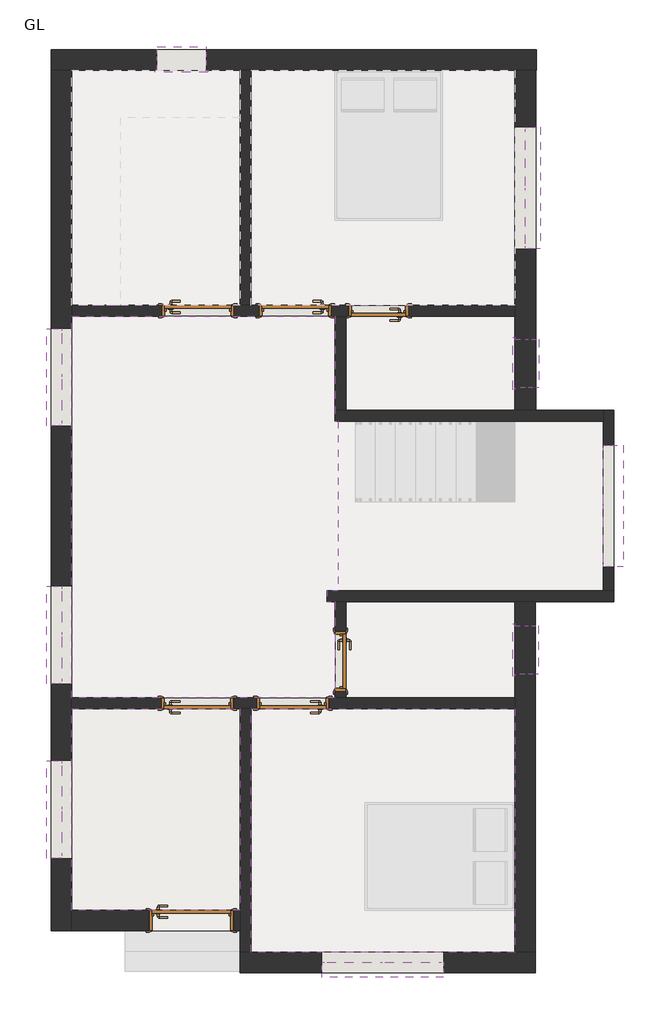
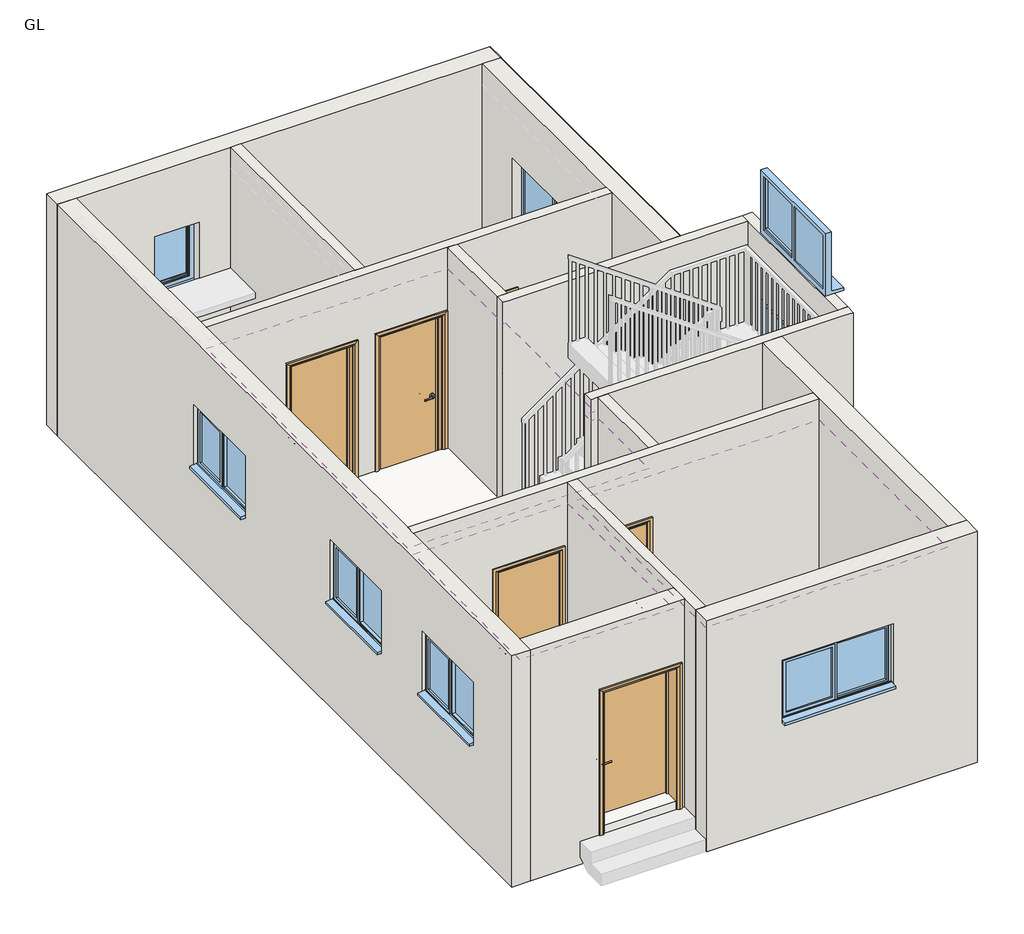
# One storey, part 1 of 3: 15 walls, 10 windows, 7 doors, 3 coverings, 1 slab.
"""IFC4 building model written with IfcOpenShell, lengths in millimetres."""

from ifc_helpers import new_model, si_unit, frame, origin, origin_with_axes, place, context, project, spatial, polyline, outline, extrude, faceted_brep, transform, mapped, element, save
from components import doors_intsgl_d1_0ae72840, doors_intsgl_d1_00c56c0f, doors_intsgl_d2_0f955423, doors_intsgl_d3_a434ac6e, windows_concept_plain_dbl_w1_41c00efb, windows_concept_plain_dbl_w2_969b2eef, windows_concept_plain_dbl_w5_831b8d9f, windows_concept_plain_dbl_w5_572de7b6, windows_sgl_plain_w3_3107c001, windows_sgl_plain_w4_5502dfe6, windows_sgl_plain_w4_0cd65ee0

model = new_model("IFC4")

# Units and contexts
model_context = context("Model", 3, world=origin())
ifc_project = project(units=[si_unit("LENGTHUNIT", "METRE", prefix="MILLI")], contexts=[model_context])

# Site, building, storey
site = spatial("IfcSite", under=ifc_project)
building = spatial("IfcBuilding", under=site)
storey = spatial("IfcBuildingStorey", under=building, Name="GL", Elevation=0.0)

# Coverings
placement = place(None, origin())
element("IfcCovering", 1, ObjectType="Plain", at=placement, inside=storey, context=model_context, shape_type="SweptSolid", body=[
    extrude(outline(polyline([(-2560.7974044, 3978.0303577), (-5865.3374044, 3978.0303577), (-5865.3374044, 8762.2021562), (-2558.2574044, 8762.2021562), (-2558.2574044, 7446.2287671), (-2525.4108818, 7446.2287671), (-2525.4108818, 5317.8803577), (-2662.3974044, 5317.8803577), (-2662.3974044, 5180.7203577), (-2560.7974044, 5180.7203577), (-2560.7974044, 3978.0303577)])), frame((0.0, 0.0, 2743.2), z_axis=(0.0, 0.0, 1.0), x_axis=(1.0, 0.0, 0.0)), (0.0, 0.0, 1.0), 57.0),
])
element("IfcCovering", 2, ObjectType="Plain", at=placement, inside=storey, context=model_context, shape_type="SweptSolid", body=[
    extrude(outline(polyline([(-3754.5974044, 1313.5703577), (-5865.3374044, 1313.5703577), (-5865.3374044, 3840.8703577), (-3754.5974044, 3840.8703577), (-3754.5974044, 1313.5703577)])), frame((0.0, 0.0, 2743.2), z_axis=(0.0, 0.0, 1.0), x_axis=(1.0, 0.0, 0.0)), (0.0, 0.0, 1.0), 57.0),
])
element("IfcCovering", 3, ObjectType="Plain", at=placement, inside=storey, context=model_context, shape_type="SweptSolid", body=[
    extrude(outline(polyline([(-301.4674044, 3840.8703577), (-301.4674044, 786.2154997), (-3617.4374044, 786.2154997), (-3617.4374044, 3840.8703577), (-301.4674044, 3840.8703577)])), frame((0.0, 0.0, 2743.2), z_axis=(0.0, 0.0, 1.0), x_axis=(1.0, 0.0, 0.0)), (0.0, 0.0, 1.0), 57.0),
])

# Doors
doors_intsgl_d1_shape = doors_intsgl_d1_0ae72840(model_context)
element("IfcDoor", 4, ObjectType="Doors_IntSgl : D1", at=placement, inside=storey, context=model_context, shape_type="MappedRepresentation", body=[
    mapped(doors_intsgl_d1_shape, transform((-4282.9174044, 8830.7821562, 0.0), x_axis=(1.0, 0.0, 0.0), y_axis=(0.0, 1.0, 0.0), z_axis=(0.0, 0.0, 1.0))),
])
element("IfcDoor", 5, ObjectType="Doors_IntSgl : D1", at=placement, inside=storey, context=model_context, shape_type="MappedRepresentation", body=[
    mapped(doors_intsgl_d1_shape, transform((-3089.1174044, 3909.4503577, 0.0), x_axis=(-1.0, 0.0, 0.0), y_axis=(0.0, -1.0, 0.0), z_axis=(0.0, 0.0, 1.0))),
])
doors_intsgl_d1_2_shape = doors_intsgl_d1_00c56c0f(model_context)
element("IfcDoor", 6, ObjectType="Doors_IntSgl : D1", at=placement, inside=storey, context=model_context, shape_type="MappedRepresentation", body=[
    mapped(doors_intsgl_d1_2_shape, transform((-3059.9079594, 8830.7821562, 0.2374744), x_axis=(-1.0, 0.0, 0.0), y_axis=(0.0, -1.0, 0.0), z_axis=(0.0, 0.0, 1.0))),
])
element("IfcDoor", 7, ObjectType="Doors_IntSgl : D1", at=placement, inside=storey, context=model_context, shape_type="MappedRepresentation", body=[
    mapped(doors_intsgl_d1_2_shape, transform((-4287.9974044, 3909.4503577, 0.0), x_axis=(1.0, 0.0, 0.0), y_axis=(0.0, 1.0, 0.0), z_axis=(0.0, 0.0, 1.0))),
])
doors_intsgl_d2_shape = doors_intsgl_d2_0f955423(model_context)
element("IfcDoor", 8, ObjectType="Doors_IntSgl : D2", at=placement, inside=storey, context=model_context, shape_type="MappedRepresentation", body=[
    mapped(doors_intsgl_d2_shape, transform((-4364.1974044, 1184.0303577, 0.0), x_axis=(1.0, 0.0, 0.0), y_axis=(0.0, 1.0, 0.0), z_axis=(0.0, 0.0, 1.0))),
])
doors_intsgl_d3_shape = doors_intsgl_d3_a434ac6e(model_context)
element("IfcDoor", 9, ObjectType="Doors_IntSgl : D3", at=placement, inside=storey, context=model_context, shape_type="MappedRepresentation", body=[
    mapped(doors_intsgl_d3_shape, transform((-2492.2174044, 4435.2303577, 0.0), x_axis=(0.0, -1.0, 0.0), y_axis=(1.0, 0.0, 0.0), z_axis=(0.0, 0.0, 1.0))),
])
element("IfcDoor", 10, ObjectType="Doors_IntSgl : D3", at=placement, inside=storey, context=model_context, shape_type="MappedRepresentation", body=[
    mapped(doors_intsgl_d3_shape, transform((-2014.6974044, 8830.7821562, 0.0), x_axis=(-1.0, 0.0, 0.0), y_axis=(0.0, -1.0, 0.0), z_axis=(0.0, 0.0, 1.0))),
])

# Slab
element("IfcSlab", 11, ObjectType="DRAWING AREA", at=placement, inside=storey, context=model_context, shape_type="SweptSolid", body=[
    extrude(outline(polyline([(-3754.5974044, 3840.8703577), (-3754.5974044, 1054.4903577), (-4897.5974044, 1054.4903577), (-4897.5974044, 1313.5703577), (-5865.3374044, 1313.5703577), (-5865.3374044, 3840.8703577), (-3754.5974044, 3840.8703577)])), origin_with_axes(), (0.0, 0.0, 1.0), 149.9616),
])

# Walls
element("IfcWall", 12, ObjectType="EX WALL", at=placement, inside=storey, context=model_context, shape_type="Brep", body=[
    faceted_brep([(-6124.4174044, 11850.4554997, -304.8), (-5865.3374044, 11850.4554997, -304.8), (-3749.5174044, 11850.4554997, -304.8), (-3612.3574044, 11850.4554997, -304.8), (-299.7708818, 11850.4554997, -304.8), (-40.6908818, 11850.4554997, -304.8), (-35.9908931, 11850.4554997, -304.8), (-35.9908931, 11850.4554997, 3048.0), (-40.6908818, 11850.4554997, 3048.0), (-42.3874044, 11850.4554997, 3048.0), (-299.7708818, 11850.4554997, 3048.0), (-3612.3574044, 11850.4554997, 3048.0), (-3749.5174044, 11850.4554997, 3048.0), (-5865.3374044, 11850.4554997, 3048.0), (-6124.4174044, 11850.4554997, 3048.0), (-4790.9174044, 11850.4554997, 2110.0), (-4181.3174044, 11850.4554997, 2110.0), (-4181.3174044, 11850.4554997, 1200.0), (-4790.9174044, 11850.4554997, 1200.0), (-6124.4174044, 12109.5354997, -304.8), (-6124.4174044, 12109.5354997, 3048.0), (-42.3874044, 12109.5354997, 3048.0), (-35.9908931, 12109.5354997, 3048.0), (-35.9908931, 12109.5354997, -304.8), (-4790.9174044, 12109.5354997, 2110.0), (-4790.9174044, 12109.5354997, 1200.0), (-4181.3174044, 12109.5354997, 1200.0), (-4181.3174044, 12109.5354997, 2110.0)], [[[0, 1, 2, 3, 4, 5, 6, 7, 8, 9, 10, 11, 12, 13, 14], [15, 16, 17, 18]], [[19, 20, 21, 22, 23], [24, 25, 26, 27]], [[6, 5, 4, 3, 2, 1, 0, 19, 23]], [[7, 6, 23, 22]], [[0, 14, 20, 19]], [[25, 24, 15, 18]], [[26, 25, 18, 17]], [[27, 26, 17, 16]], [[24, 27, 16, 15]], [[9, 8, 7, 22, 21]], [[14, 13, 12, 11, 10, 9, 21, 20]]]),
])
element("IfcWall", 13, ObjectType="EX WALL", at=placement, inside=storey, context=model_context, shape_type="Brep", body=[
    faceted_brep([(-5865.3374044, 1054.4903577, -304.8), (-5865.3374044, 1313.5703577, -304.8), (-5865.3374044, 3840.8703577, -304.8), (-5865.3374044, 3978.0303577, -304.8), (-5865.3374044, 8762.2021562, -304.8), (-5865.3374044, 8899.3621562, -304.8), (-5865.3374044, 11850.4554997, -304.8), (-5865.3374044, 11850.4554997, 3048.0), (-5865.3374044, 8899.3621562, 3048.0), (-5865.3374044, 8762.2021562, 3048.0), (-5865.3374044, 3978.0303577, 3048.0), (-5865.3374044, 3840.8703577, 3048.0), (-5865.3374044, 1313.5703577, 3048.0), (-5865.3374044, 1054.4903577, 3048.0), (-5865.3374044, 1967.6203577, 2110.0), (-5865.3374044, 3186.8203577, 2110.0), (-5865.3374044, 3186.8203577, 1200.0), (-5865.3374044, 1967.6203577, 1200.0), (-5865.3374044, 4155.8303577, 2110.0), (-5865.3374044, 5375.0303577, 2110.0), (-5865.3374044, 5375.0303577, 1200.0), (-5865.3374044, 4155.8303577, 1200.0), (-5865.3374044, 7390.6021562, 2110.0), (-5865.3374044, 8609.8021562, 2110.0), (-5865.3374044, 8609.8021562, 1200.0), (-5865.3374044, 7390.6021562, 1200.0), (-6124.4174044, 1054.4903577, -304.8), (-6124.4174044, 1054.4903577, 3048.0), (-6124.4174044, 11850.4554997, 3048.0), (-6124.4174044, 11850.4554997, -304.8), (-6124.4174044, 1967.6203577, 2110.0), (-6124.4174044, 1967.6203577, 1200.0), (-6124.4174044, 3186.8203577, 1200.0), (-6124.4174044, 3186.8203577, 2110.0), (-6124.4174044, 4155.8303577, 2110.0), (-6124.4174044, 4155.8303577, 1200.0), (-6124.4174044, 5375.0303577, 1200.0), (-6124.4174044, 5375.0303577, 2110.0), (-6124.4174044, 7390.6021562, 2110.0), (-6124.4174044, 7390.6021562, 1200.0), (-6124.4174044, 8609.8021562, 1200.0), (-6124.4174044, 8609.8021562, 2110.0)], [[[0, 1, 2, 3, 4, 5, 6, 7, 8, 9, 10, 11, 12, 13], [14, 15, 16, 17], [18, 19, 20, 21], [22, 23, 24, 25]], [[26, 27, 28, 29], [30, 31, 32, 33], [34, 35, 36, 37], [38, 39, 40, 41]], [[6, 5, 4, 3, 2, 1, 0, 26, 29]], [[7, 6, 29, 28]], [[0, 13, 27, 26]], [[31, 30, 14, 17]], [[32, 31, 17, 16]], [[33, 32, 16, 15]], [[30, 33, 15, 14]], [[35, 34, 18, 21]], [[36, 35, 21, 20]], [[37, 36, 20, 19]], [[34, 37, 19, 18]], [[39, 38, 22, 25]], [[40, 39, 25, 24]], [[41, 40, 24, 23]], [[38, 41, 23, 22]], [[13, 12, 11, 10, 9, 8, 7, 28, 27]]]),
])
element("IfcWall", 14, ObjectType="EX WALL", at=placement, inside=storey, context=model_context, shape_type="SweptSolid", body=[
    extrude(outline(polyline([(-304.8, -5865.3374044), (-304.8, -3754.5974044), (3048.0, -3754.5974044), (3048.0, -5865.3374044), (-304.8, -5865.3374044)]), holes=[polyline([(2110.0, -3830.7974044), (0.0, -3830.7974044), (0.0, -4897.5974044), (2110.0, -4897.5974044), (2110.0, -3830.7974044)])]), frame((0.0, 1054.4903577, 0.0), z_axis=(0.0, 1.0, 0.0), x_axis=(0.0, 0.0, 1.0)), (0.0, 0.0, 1.0), 259.08),
])
element("IfcWall", 15, ObjectType="EX WALL", at=placement, inside=storey, context=model_context, shape_type="Brep", body=[
    faceted_brep([(-3754.5974044, 527.1354997, -304.8), (-42.3874044, 527.1354997, -304.8), (-42.3874044, 527.1354997, 3048.0), (-3754.5974044, 527.1354997, 3048.0), (-1197.4524044, 527.1354997, 2110.0), (-1197.4524044, 527.1354997, 1200.0), (-2721.4524044, 527.1354997, 1200.0), (-2721.4524044, 527.1354997, 2110.0), (-3754.5974044, 786.2154997, -304.8), (-3754.5974044, 786.2154997, 3048.0), (-3617.4374044, 786.2154997, 3048.0), (-301.4674044, 786.2154997, 3048.0), (-42.3874044, 786.2154997, 3048.0), (-42.3874044, 786.2154997, -304.8), (-301.4674044, 786.2154997, -304.8), (-3617.4374044, 786.2154997, -304.8), (-1197.4524044, 786.2154997, 2110.0), (-2721.4524044, 786.2154997, 2110.0), (-2721.4524044, 786.2154997, 1200.0), (-1197.4524044, 786.2154997, 1200.0)], [[[0, 1, 2, 3], [4, 5, 6, 7]], [[8, 9, 10, 11, 12, 13, 14, 15], [16, 17, 18, 19]], [[1, 0, 8, 15, 14, 13]], [[2, 1, 13, 12]], [[0, 3, 9, 8]], [[5, 4, 16, 19]], [[6, 5, 19, 18]], [[7, 6, 18, 17]], [[4, 7, 17, 16]], [[3, 2, 12, 11, 10, 9]]]),
])
element("IfcWall", 16, ObjectType="EX WALL", at=placement, inside=storey, context=model_context, shape_type="Brep", body=[
    faceted_brep([(-42.3874044, 786.2154997, -304.8), (-42.3874044, 5180.7203577, -304.8), (-42.3874044, 5180.7203577, 3048.0), (-42.3874044, 786.2154997, 3048.0), (-42.3874044, 4274.5753577, 2133.6), (-42.3874044, 4884.1753577, 2133.6), (-42.3874044, 4884.1753577, 1524.0), (-42.3874044, 4274.5753577, 1524.0), (-301.4674044, 786.2154997, -304.8), (-301.4674044, 786.2154997, 3048.0), (-301.4674044, 3840.8703577, 3048.0), (-301.4674044, 3978.0303577, 3048.0), (-301.4674044, 5180.7203577, 3048.0), (-301.4674044, 5180.7203577, -304.8), (-301.4674044, 3978.0303577, -304.8), (-301.4674044, 3840.8703577, -304.8), (-301.4674044, 4274.5753577, 2133.6), (-301.4674044, 4274.5753577, 1524.0), (-301.4674044, 4884.1753577, 1524.0), (-301.4674044, 4884.1753577, 2133.6)], [[[0, 1, 2, 3], [4, 5, 6, 7]], [[8, 9, 10, 11, 12, 13, 14, 15], [16, 17, 18, 19]], [[1, 0, 8, 15, 14, 13]], [[0, 3, 9, 8]], [[17, 16, 4, 7]], [[18, 17, 7, 6]], [[19, 18, 6, 5]], [[16, 19, 5, 4]], [[3, 2, 12, 11, 10, 9]], [[1, 13, 12, 2]]]),
])
element("IfcWall", 17, ObjectType="EX WALL", at=placement, inside=storey, context=model_context, shape_type="Brep", body=[
    faceted_brep([(-40.6908818, 7583.3887671, 3048.0), (-40.6908818, 7583.3887671, -304.8), (-40.6908818, 11850.4554997, -304.8), (-40.6908818, 11850.4554997, 3048.0), (-40.6908818, 11136.9088279, 2110.0), (-40.6908818, 11136.9088279, 1200.0), (-40.6908818, 9612.9088279, 1200.0), (-40.6908818, 9612.9088279, 2110.0), (-40.6908818, 8477.5954616, 2133.6), (-40.6908818, 8477.5954616, 1524.0), (-40.6908818, 7867.9954616, 1524.0), (-40.6908818, 7867.9954616, 2133.6), (-299.7708818, 7583.3887671, -304.8), (-299.7708818, 7583.3887671, 3048.0), (-299.7708818, 8762.2021562, 3048.0), (-299.7708818, 8899.3621562, 3048.0), (-299.7708818, 11850.4554997, 3048.0), (-299.7708818, 11850.4554997, -304.8), (-299.7708818, 8899.3621562, -304.8), (-299.7708818, 8762.2021562, -304.8), (-299.7708818, 11136.9088279, 2110.0), (-299.7708818, 9612.9088279, 2110.0), (-299.7708818, 9612.9088279, 1200.0), (-299.7708818, 11136.9088279, 1200.0), (-299.7708818, 8477.5954616, 2133.6), (-299.7708818, 7867.9954616, 2133.6), (-299.7708818, 7867.9954616, 1524.0), (-299.7708818, 8477.5954616, 1524.0), (-42.3874044, 11850.4554997, 3048.0), (-42.3874044, 7583.3887671, 3048.0)], [[[0, 1, 2, 3], [4, 5, 6, 7], [8, 9, 10, 11]], [[12, 13, 14, 15, 16, 17, 18, 19], [20, 21, 22, 23], [24, 25, 26, 27]], [[2, 1, 12, 19, 18, 17]], [[3, 2, 17, 16, 28]], [[5, 4, 20, 23]], [[6, 5, 23, 22]], [[7, 6, 22, 21]], [[4, 7, 21, 20]], [[9, 8, 24, 27]], [[10, 9, 27, 26]], [[11, 10, 26, 25]], [[8, 11, 25, 24]], [[0, 3, 28, 29]], [[28, 16, 15, 14, 13, 29]], [[0, 29, 13, 12, 1]]]),
])
element("IfcWall", 18, ObjectType="INNER WALL", at=placement, inside=storey, context=model_context, shape_type="Brep", body=[
    faceted_brep([(-3617.4374044, 786.2154997, -304.8), (-3617.4374044, 3840.8703577, -304.8), (-3617.4374044, 3840.8703577, 3048.0), (-3617.4374044, 786.2154997, 3048.0), (-3754.5974044, 786.2154997, -304.8), (-3754.5974044, 786.2154997, 3048.0), (-3754.5974044, 1054.4903577, 3048.0), (-3754.5974044, 1313.5703577, 3048.0), (-3754.5974044, 3840.8703577, 3048.0), (-3754.5974044, 3840.8703577, -304.8), (-3754.5974044, 1313.5703577, -304.8), (-3754.5974044, 1054.4903577, -304.8)], [[[0, 1, 2, 3]], [[4, 5, 6, 7, 8, 9, 10, 11]], [[1, 0, 4, 11, 10, 9]], [[0, 3, 5, 4]], [[2, 1, 9, 8]], [[3, 2, 8, 7, 6, 5]]]),
])
element("IfcWall", 19, ObjectType="INNER WALL", at=placement, inside=storey, context=model_context, shape_type="Brep", body=[
    faceted_brep([(-5865.3374044, 3840.8703577, -304.8), (-3754.5974044, 3840.8703577, -304.8), (-3617.4374044, 3840.8703577, -304.8), (-301.4674044, 3840.8703577, -304.8), (-301.4674044, 3840.8703577, 3048.0), (-3617.4374044, 3840.8703577, 3048.0), (-3754.5974044, 3840.8703577, 3048.0), (-5865.3374044, 3840.8703577, 3048.0), (-3546.3174044, 3840.8703577, 0.0), (-3546.3174044, 3840.8703577, 2110.0), (-2631.9174044, 3840.8703577, 2110.0), (-2631.9174044, 3840.8703577, 0.0), (-3830.7974044, 3840.8703577, 2110.0), (-3830.7974044, 3840.8703577, 0.0), (-4745.1974044, 3840.8703577, 0.0), (-4745.1974044, 3840.8703577, 2110.0), (-301.4674044, 3978.0303577, -304.8), (-2423.6374044, 3978.0303577, -304.8), (-2560.7974044, 3978.0303577, -304.8), (-5865.3374044, 3978.0303577, -304.8), (-5865.3374044, 3978.0303577, 3048.0), (-2560.7974044, 3978.0303577, 3048.0), (-2423.6374044, 3978.0303577, 3048.0), (-301.4674044, 3978.0303577, 3048.0), (-3546.3174044, 3978.0303577, 2110.0), (-3546.3174044, 3978.0303577, 0.0), (-2631.9174044, 3978.0303577, 0.0), (-2631.9174044, 3978.0303577, 2110.0), (-3830.7974044, 3978.0303577, 0.0), (-3830.7974044, 3978.0303577, 2110.0), (-4745.1974044, 3978.0303577, 2110.0), (-4745.1974044, 3978.0303577, 0.0)], [[[0, 1, 2, 3, 4, 5, 6, 7], [8, 9, 10, 11], [12, 13, 14, 15]], [[16, 17, 18, 19, 20, 21, 22, 23], [24, 25, 26, 27], [28, 29, 30, 31]], [[3, 2, 1, 0, 19, 18, 17, 16]], [[0, 7, 20, 19]], [[4, 3, 16, 23]], [[8, 25, 24, 9]], [[9, 24, 27, 10]], [[10, 27, 26, 11]], [[25, 8, 11, 26]], [[28, 13, 12, 29]], [[29, 12, 15, 30]], [[14, 31, 30, 15]], [[13, 28, 31, 14]], [[7, 6, 5, 4, 23, 22, 21, 20]]]),
])
element("IfcWall", 20, ObjectType="INNER WALL", at=placement, inside=storey, context=model_context, shape_type="SweptSolid", body=[
    extrude(outline(polyline([(5180.7203577, -304.8), (3978.0303577, -304.8), (3978.0303577, 3048.0), (5180.7203577, 3048.0), (5180.7203577, -304.8)]), holes=[polyline([(4054.2303577, 2110.0), (4054.2303577, 0.0), (4816.2303577, 0.0), (4816.2303577, 2110.0), (4054.2303577, 2110.0)])]), frame((-2560.7974044, 0.0, 0.0), z_axis=(1.0, 0.0, 0.0), x_axis=(0.0, 1.0, 0.0)), (0.0, 0.0, 1.0), 137.16),
])
element("IfcWall", 21, ObjectType="INNER WALL", at=placement, inside=storey, context=model_context, shape_type="Brep", body=[
    faceted_brep([(-2662.3974044, 5180.7203577, -304.8), (-2560.7974044, 5180.7203577, -304.8), (-2423.6374044, 5180.7203577, -304.8), (-301.4674044, 5180.7203577, -304.8), (-42.3874044, 5180.7203577, -304.8), (941.6891182, 5180.7203577, -304.8), (941.6891182, 5180.7203577, 3048.0), (804.5291182, 5180.7203577, 3048.0), (-42.3874044, 5180.7203577, 3048.0), (-301.4674044, 5180.7203577, 3048.0), (-2423.6374044, 5180.7203577, 3048.0), (-2560.7974044, 5180.7203577, 3048.0), (-2662.3974044, 5180.7203577, 3048.0), (-2662.3974044, 5317.8803577, -304.8), (-2662.3974044, 5317.8803577, 3048.0), (804.5291182, 5317.8803577, 3048.0), (941.6891182, 5317.8803577, 3048.0), (941.6891182, 5317.8803577, 2743.2), (941.6891182, 5317.8803577, -304.8), (804.5291182, 5317.8803577, -304.8)], [[[0, 1, 2, 3, 4, 5, 6, 7, 8, 9, 10, 11, 12]], [[13, 14, 15, 16, 17, 18, 19]], [[5, 4, 3, 2, 1, 0, 13, 19, 18]], [[0, 12, 14, 13]], [[12, 11, 10, 9, 8, 7, 6, 16, 15, 14]], [[5, 18, 17, 16, 6]]]),
])
element("IfcWall", 22, ObjectType="INNER WALL", at=placement, inside=storey, context=model_context, shape_type="Brep", body=[
    faceted_brep([(941.6891182, 5317.8803577, 3048.0), (941.6891182, 5317.8803577, -304.8), (941.6891182, 7583.3887671, -304.8), (941.6891182, 7583.3887671, 3048.0), (941.6891182, 7446.2287671, 3048.0), (941.6891182, 7144.0545624, 2110.0), (941.6891182, 7144.0545624, 1200.0), (941.6891182, 5620.0545624, 1200.0), (941.6891182, 5620.0545624, 2110.0), (804.5291182, 5317.8803577, -304.8), (804.5291182, 5317.8803577, 3048.0), (804.5291182, 7446.2287671, 3048.0), (804.5291182, 7583.3887671, 3048.0), (804.5291182, 7583.3887671, 2743.2), (804.5291182, 7583.3887671, -304.8), (804.5291182, 7446.2287671, -304.8), (804.5291182, 7144.0545624, 2110.0), (804.5291182, 5620.0545624, 2110.0), (804.5291182, 5620.0545624, 1200.0), (804.5291182, 7144.0545624, 1200.0)], [[[0, 1, 2, 3, 4], [5, 6, 7, 8]], [[9, 10, 11, 12, 13, 14, 15], [16, 17, 18, 19]], [[2, 1, 9, 15, 14]], [[0, 4, 3, 12, 11, 10]], [[6, 5, 16, 19]], [[7, 6, 19, 18]], [[8, 7, 18, 17]], [[5, 8, 17, 16]], [[2, 14, 13, 12, 3]], [[0, 10, 9, 1]]]),
])
element("IfcWall", 23, ObjectType="INNER WALL", at=placement, inside=storey, context=model_context, shape_type="Brep", body=[
    faceted_brep([(804.5291182, 7583.3887671, 3048.0), (804.5291182, 7583.3887671, -304.8), (-40.6908818, 7583.3887671, -304.8), (-299.7708818, 7583.3887671, -304.8), (-2421.0974044, 7583.3887671, -304.8), (-2558.2574044, 7583.3887671, -304.8), (-2558.2574044, 7583.3887671, 3048.0), (-2459.1974044, 7583.3887671, 3048.0), (-2421.0974044, 7583.3887671, 3048.0), (-299.7708818, 7583.3887671, 3048.0), (-42.3874044, 7583.3887671, 3048.0), (-40.6908818, 7583.3887671, 3048.0), (804.5291182, 7446.2287671, -304.8), (804.5291182, 7446.2287671, 3048.0), (-2421.0974044, 7446.2287671, 3048.0), (-2459.1974044, 7446.2287671, 3048.0), (-2558.2574044, 7446.2287671, 3048.0), (-2558.2574044, 7446.2287671, -304.8)], [[[0, 1, 2, 3, 4, 5, 6, 7, 8, 9, 10, 11]], [[12, 13, 14, 15, 16, 17]], [[5, 4, 3, 2, 1, 12, 17]], [[0, 11, 10, 9, 8, 7, 6, 16, 15, 14, 13]], [[5, 17, 16, 6]], [[0, 13, 12, 1]]]),
])
element("IfcWall", 24, ObjectType="INNER WALL", at=placement, inside=storey, context=model_context, shape_type="Brep", body=[
    faceted_brep([(-2421.0974044, 7583.3887671, -304.8), (-2421.0974044, 8762.2021562, -304.8), (-2421.0974044, 8762.2021562, 3048.0), (-2421.0974044, 7583.3887671, 3048.0), (-2558.2574044, 8762.2021562, -304.8), (-2558.2574044, 7583.3887671, -304.8), (-2558.2574044, 7583.3887671, 0.0), (-2558.2574044, 7583.3887671, 149.9616), (-2558.2574044, 7583.3887671, 3048.0), (-2558.2574044, 8762.2021562, 3048.0), (-2558.2574044, 8762.2021562, 149.9616), (-2558.2574044, 8762.2021562, 0.0)], [[[0, 1, 2, 3]], [[4, 5, 6, 7, 8, 9, 10, 11]], [[1, 0, 5, 4]], [[2, 1, 4, 11, 10, 9]], [[3, 2, 9, 8]], [[5, 0, 3, 8, 7, 6]]]),
])
element("IfcWall", 25, ObjectType="INNER WALL", at=placement, inside=storey, context=model_context, shape_type="Brep", body=[
    faceted_brep([(-5865.3374044, 8762.2021562, -304.8), (-2558.2574044, 8762.2021562, -304.8), (-2421.0974044, 8762.2021562, -304.8), (-299.7708818, 8762.2021562, -304.8), (-299.7708818, 8762.2021562, 3048.0), (-2421.0974044, 8762.2021562, 3048.0), (-2558.2574044, 8762.2021562, 3048.0), (-5865.3374044, 8762.2021562, 3048.0), (-3825.7174044, 8762.2021562, 2110.0), (-3825.7174044, 8762.2021562, 0.0), (-4740.1174044, 8762.2021562, 0.0), (-4740.1174044, 8762.2021562, 2110.0), (-3517.1079594, 8762.2021562, 0.2374744), (-3517.1079594, 8762.2021562, 2110.2374744), (-2602.7079594, 8762.2021562, 2110.2374744), (-2602.7079594, 8762.2021562, 0.2374744), (-2395.6974044, 8762.2021562, 0.0), (-2395.6974044, 8762.2021562, 2110.0), (-1633.6974044, 8762.2021562, 2110.0), (-1633.6974044, 8762.2021562, 0.0), (-299.7708818, 8899.3621562, -304.8), (-3612.3574044, 8899.3621562, -304.8), (-3749.5174044, 8899.3621562, -304.8), (-5865.3374044, 8899.3621562, -304.8), (-5865.3374044, 8899.3621562, 0.0), (-5865.3374044, 8899.3621562, 149.9616), (-5865.3374044, 8899.3621562, 3048.0), (-3749.5174044, 8899.3621562, 3048.0), (-3612.3574044, 8899.3621562, 3048.0), (-299.7708818, 8899.3621562, 3048.0), (-3825.7174044, 8899.3621562, 0.0), (-3825.7174044, 8899.3621562, 2110.0), (-4740.1174044, 8899.3621562, 2110.0), (-4740.1174044, 8899.3621562, 0.0), (-3517.1079594, 8899.3621562, 2110.2374744), (-3517.1079594, 8899.3621562, 0.2374744), (-2602.7079594, 8899.3621562, 0.2374744), (-2602.7079594, 8899.3621562, 2110.2374744), (-2395.6974044, 8899.3621562, 2110.0), (-2395.6974044, 8899.3621562, 0.0), (-1633.6974044, 8899.3621562, 0.0), (-1633.6974044, 8899.3621562, 2110.0)], [[[0, 1, 2, 3, 4, 5, 6, 7], [8, 9, 10, 11], [12, 13, 14, 15], [16, 17, 18, 19]], [[20, 21, 22, 23, 24, 25, 26, 27, 28, 29], [30, 31, 32, 33], [34, 35, 36, 37], [38, 39, 40, 41]], [[3, 2, 1, 0, 23, 22, 21, 20]], [[0, 7, 26, 25, 24, 23]], [[4, 3, 20, 29]], [[30, 9, 8, 31]], [[31, 8, 11, 32]], [[32, 11, 10, 33]], [[9, 30, 33, 10]], [[12, 35, 34, 13]], [[13, 34, 37, 14]], [[36, 15, 14, 37]], [[35, 12, 15, 36]], [[16, 39, 38, 17]], [[17, 38, 41, 18]], [[40, 19, 18, 41]], [[39, 16, 19, 40]], [[7, 6, 5, 4, 29, 28, 27, 26]]]),
])
element("IfcWall", 26, ObjectType="INNER WALL", at=placement, inside=storey, context=model_context, shape_type="SweptSolid", body=[
    extrude(outline(polyline([(-3612.3574044, 11850.4554997), (-3612.3574044, 8899.3621562), (-3749.5174044, 8899.3621562), (-3749.5174044, 11850.4554997), (-3612.3574044, 11850.4554997)])), frame((0.0, 0.0, -304.8), z_axis=(0.0, 0.0, 1.0), x_axis=(1.0, 0.0, 0.0)), (0.0, 0.0, 1.0), 3352.8),
])

# Windows
windows_concept_plain_dbl_w1_shape = windows_concept_plain_dbl_w1_41c00efb(model_context)
element("IfcWindow", 27, ObjectType="Windows_Concept_Plain_Dbl : W1", at=placement, inside=storey, context=model_context, shape_type="MappedRepresentation", body=[
    mapped(windows_concept_plain_dbl_w1_shape, transform((-5986.4208366, 2862.2203577, 0.0), x_axis=(0.0, 1.0, 0.0), y_axis=(-1.0, 0.0, 0.0), z_axis=(0.0, 0.0, 1.0))),
])
element("IfcWindow", 28, ObjectType="Windows_Concept_Plain_Dbl : W1", at=placement, inside=storey, context=model_context, shape_type="MappedRepresentation", body=[
    mapped(windows_concept_plain_dbl_w1_shape, transform((-5986.4208366, 5050.4303577, 0.0), x_axis=(0.0, 1.0, 0.0), y_axis=(-1.0, 0.0, 0.0), z_axis=(0.0, 0.0, 1.0))),
])
element("IfcWindow", 29, ObjectType="Windows_Concept_Plain_Dbl : W1", at=placement, inside=storey, context=model_context, shape_type="MappedRepresentation", body=[
    mapped(windows_concept_plain_dbl_w1_shape, transform((-5986.4208366, 8285.2021562, 0.0), x_axis=(0.0, 1.0, 0.0), y_axis=(-1.0, 0.0, 0.0), z_axis=(0.0, 0.0, 1.0))),
])
windows_concept_plain_dbl_w2_shape = windows_concept_plain_dbl_w2_969b2eef(model_context)
element("IfcWindow", 30, ObjectType="Windows_Concept_Plain_Dbl : W2", at=placement, inside=storey, context=model_context, shape_type="MappedRepresentation", body=[
    mapped(windows_concept_plain_dbl_w2_shape, transform((-2244.4524044, 665.1320675, 0.0), x_axis=(-1.0, 0.0, 0.0), y_axis=(0.0, -1.0, 0.0), z_axis=(0.0, 0.0, 1.0))),
])
element("IfcWindow", 31, ObjectType="Windows_Concept_Plain_Dbl : W2", at=placement, inside=storey, context=model_context, shape_type="MappedRepresentation", body=[
    mapped(windows_concept_plain_dbl_w2_shape, transform((-178.6874496, 10089.9088279, 0.0), x_axis=(0.0, -1.0, 0.0), y_axis=(1.0, 0.0, 0.0), z_axis=(0.0, 0.0, 1.0))),
])
windows_concept_plain_dbl_w5_shape = windows_concept_plain_dbl_w5_831b8d9f(model_context)
element("IfcWindow", 32, ObjectType="Windows_Concept_Plain_Dbl : W5", at=placement, inside=storey, context=model_context, shape_type="MappedRepresentation", body=[
    mapped(windows_concept_plain_dbl_w5_shape, transform((864.6525504, 6097.0545624, 0.0), x_axis=(0.0, -1.0, 0.0), y_axis=(1.0, 0.0, 0.0), z_axis=(0.0, 0.0, 1.0))),
])
windows_concept_plain_dbl_w5_2_shape = windows_concept_plain_dbl_w5_572de7b6(model_context)
element("IfcWindow", 33, ObjectType="Windows_Concept_Plain_Dbl : W5", at=placement, inside=storey, context=model_context, shape_type="MappedRepresentation", body=[
    mapped(windows_concept_plain_dbl_w5_2_shape, transform((864.6525504, 6667.0545624, 1864.1348707), x_axis=(0.0, 1.0, 0.0), y_axis=(-1.0, 0.0, 0.0), z_axis=(0.0, 0.0, 1.0))),
])
windows_sgl_plain_w3_shape = windows_sgl_plain_w3_3107c001(model_context)
element("IfcWindow", 34, ObjectType="Windows_Sgl_Plain : W3", at=placement, inside=storey, context=model_context, shape_type="MappedRepresentation", body=[
    mapped(windows_sgl_plain_w3_shape, transform((-4486.1174044, 11971.5389318, 0.0), x_axis=(1.0, 0.0, 0.0), y_axis=(0.0, 1.0, 0.0), z_axis=(0.0, 0.0, 1.0))),
])
windows_sgl_plain_w4_shape = windows_sgl_plain_w4_5502dfe6(model_context)
element("IfcWindow", 35, ObjectType="Windows_Sgl_Plain : W4", at=placement, inside=storey, context=model_context, shape_type="MappedRepresentation", body=[
    mapped(windows_sgl_plain_w4_shape, transform((-178.6874496, 8172.7954616, 23.6), x_axis=(0.0, -1.0, 0.0), y_axis=(1.0, 0.0, 0.0), z_axis=(0.0, 0.0, 1.0))),
])
windows_sgl_plain_w4_2_shape = windows_sgl_plain_w4_0cd65ee0(model_context)
element("IfcWindow", 36, ObjectType="Windows_Sgl_Plain : W4", at=placement, inside=storey, context=model_context, shape_type="MappedRepresentation", body=[
    mapped(windows_sgl_plain_w4_2_shape, transform((-180.3839722, 4579.3753577, 23.6), x_axis=(0.0, 1.0, 0.0), y_axis=(-1.0, 0.0, 0.0), z_axis=(0.0, 0.0, 1.0))),
])

save(model, "model.ifc")

# Revit data of these elements
# Type "Plain"
#   Keynote = "K40"
#   built-in parameter 1002203 = 1 (stored number, unit not read)
#   built-in parameter 1002202 = 1 (stored number, unit not read)
#   Layers, outside or top first: 45 mm "Metal Stud Layer" (function 1); 12 mm "Gypsum Wall Board" (function 1)
# Type "Doors_IntSgl : D1"
#   Type Mark = "46"
#   Type Comments = "Internal Single"
#   Operation = "SingleSwingRight"
#   Manufacturer = "Revit"
#   Keynote = "L20"
#   Description = "Internal Single Door"
#   Analytic Construction = "Metal"
#   UnderCut = 8 mm
#   Tolerance = 2 mm
#   Thickness = 38 mm
#   Thermal Resistance (R) = 0.270117 (m²·K)/W
#   Structural Tolerance = 8 mm
#   StopDepth = 32 mm
#   Stop Thickness = 19 mm
#   Rough Width = 914.4 mm
#   Rough Height = 2110 mm
#   Height to Top Lock Rail = 1000 mm
#   Heat Transfer Coefficient (U) = 3.7021 W/(m²·K)
#   Handle Z Distance = 900 mm
#   Handle X Distance = 75 mm
#   Frame Thickness = 32 mm
#   Door Panel Width = 830.4 mm
#   Door Panel Thickness = 38 mm
#   Door Panel Offset = 0 mm
#   Height = 2110 mm
#   Width = 914.4 mm
#   Door Panel Height = 2060 mm
#   Architrave Setback = 5 mm
#   Vis - Ironmongery = yes
#   Material Ironmongery = Door - Handle
#   Material Frame = Door - Frame/Mullion (1)
#   Material Door = Door - Panel
#   Material Architrave = Door - Architrave
#   Visual Light Transmittance = 0
#   Solar Heat Gain Coefficient = 0
#   Function = (empty or 0)
#   Wall Closure = (empty or 0)
# Type "Doors_IntSgl : D2"
#   Type Mark = "47"
#   Type Comments = "Internal Single"
#   Operation = "SingleSwingRight"
#   Manufacturer = "Revit"
#   Keynote = "L20"
#   Description = "Internal Single Door"
#   Analytic Construction = "Metal"
#   UnderCut = 8 mm
#   Tolerance = 2 mm
#   Thickness = 38 mm
#   Thermal Resistance (R) = 0.270117 (m²·K)/W
#   Structural Tolerance = 8 mm
#   StopDepth = 32 mm
#   Stop Thickness = 19 mm
#   Rough Width = 1066.8 mm
#   Rough Height = 2110 mm
#   Height to Top Lock Rail = 1000 mm
#   Heat Transfer Coefficient (U) = 3.7021 W/(m²·K)
#   Handle Z Distance = 900 mm
#   Handle X Distance = 75 mm
#   Frame Thickness = 32 mm
#   Door Panel Width = 982.8 mm
#   Door Panel Thickness = 38 mm
#   Door Panel Offset = 0 mm
#   Height = 2110 mm
#   Width = 1066.8 mm
#   Door Panel Height = 2060 mm
#   Architrave Setback = 5 mm
#   Vis - Ironmongery = yes
#   Material Ironmongery = Door - Handle
#   Material Frame = Door - Frame/Mullion (1)
#   Material Door = Door - Panel
#   Material Architrave = Door - Architrave
#   Visual Light Transmittance = 0
#   Solar Heat Gain Coefficient = 0
#   Function = (empty or 0)
#   Wall Closure = (empty or 0)
# Type "Doors_IntSgl : D3"
#   Type Mark = "48"
#   Type Comments = "Internal Single"
#   Operation = "SingleSwingRight"
#   Manufacturer = "Revit"
#   Keynote = "L20"
#   Description = "Internal Single Door"
#   Analytic Construction = "Metal"
#   UnderCut = 8 mm
#   Tolerance = 2 mm
#   Thickness = 38 mm
#   Thermal Resistance (R) = 0.270117 (m²·K)/W
#   Structural Tolerance = 8 mm
#   StopDepth = 32 mm
#   Stop Thickness = 19 mm
#   Rough Width = 762 mm
#   Rough Height = 2110 mm
#   Height to Top Lock Rail = 1000 mm
#   Heat Transfer Coefficient (U) = 3.7021 W/(m²·K)
#   Handle Z Distance = 900 mm
#   Handle X Distance = 75 mm
#   Frame Thickness = 32 mm
#   Door Panel Width = 678 mm
#   Door Panel Thickness = 38 mm
#   Door Panel Offset = 0 mm
#   Height = 2110 mm
#   Width = 762 mm
#   Door Panel Height = 2060 mm
#   Architrave Setback = 5 mm
#   Vis - Ironmongery = yes
#   Material Ironmongery = Door - Handle
#   Material Frame = Door - Frame/Mullion (1)
#   Material Door = Door - Panel
#   Material Architrave = Door - Architrave
#   Visual Light Transmittance = 0
#   Solar Heat Gain Coefficient = 0
#   Function = (empty or 0)
#   Wall Closure = (empty or 0)
# Type "DRAWING AREA"
#   Function = 0
#   Layers, outside or top first: 21.946 mm "Wood Sheathing, Chipboard" (function 5); 128.016 mm "Structure, Timber Joist/Rafter Layer" (function 1)
# Type "EX WALL"
#   Keynote = "F10"
#   Layers, outside or top first: 259.08 mm "Brick, Common" (function 1)
# Type "INNER WALL"
#   Keynote = "F10"
#   Layers, outside or top first: 137.16 mm "Brick, Common" (function 1)
# Type "Windows_Concept_Plain_Dbl : W1"
#   Type Mark = "56"
#   Operation = "DoublePanelVertical"
#   Construction Type Id = "GSP4R"
#   Manufacturer = "Revit"
#   Keynote = "L10"
#   Analytic Construction = "1/8 in Pilkington single glazing"
#   Visual Light Transmittance = 0.9
#   Solar Heat Gain Coefficient = 0.78
#   Rough Width = 1219.2 mm
#   Rough Height = 910 mm
#   Height = 910 mm
#   Width = 1219.2 mm
#   Heat Transfer Coefficient (U) = 3.6886 W/(m²·K)
#   FrameOffset - External = 50 mm
#   Default Head Height = 2110 mm
#   Vis - Cavity Closers = yes
#   Define Thermal Properties by = 1
#   Material Trim = Window Frame
#   Material Glass = Glass
#   Material Frame = Window Frame
#   Wall Closure = (empty or 0)
# Type "Windows_Concept_Plain_Dbl : W2"
#   Type Mark = "57"
#   Operation = "DoublePanelVertical"
#   Construction Type Id = "GSP4R"
#   Manufacturer = "Revit"
#   Keynote = "L10"
#   Analytic Construction = "1/8 in Pilkington single glazing"
#   Visual Light Transmittance = 0.9
#   Solar Heat Gain Coefficient = 0.78
#   Rough Width = 1524 mm
#   Rough Height = 910 mm
#   Height = 910 mm
#   Width = 1524 mm
#   Heat Transfer Coefficient (U) = 3.6886 W/(m²·K)
#   FrameOffset - External = 50 mm
#   Default Head Height = 2110 mm
#   Vis - Cavity Closers = yes
#   Define Thermal Properties by = 1
#   Material Trim = Window Frame
#   Material Glass = Glass
#   Material Frame = Window Frame
#   Wall Closure = (empty or 0)
# Type "Windows_Concept_Plain_Dbl : W5"
#   Type Mark = "60"
#   Operation = "DoublePanelVertical"
#   Construction Type Id = "GSP4R"
#   Manufacturer = "Revit"
#   Keynote = "L10"
#   Analytic Construction = "1/8 in Pilkington single glazing"
#   Visual Light Transmittance = 0.9
#   Solar Heat Gain Coefficient = 0.78
#   Rough Width = 1524 mm
#   Rough Height = 910 mm
#   Height = 910 mm
#   Width = 1524 mm
#   Heat Transfer Coefficient (U) = 3.6886 W/(m²·K)
#   FrameOffset - External = 50 mm
#   Default Head Height = 2110 mm
#   Vis - Cavity Closers = yes
#   Define Thermal Properties by = 1
#   Material Trim = Window Frame
#   Material Glass = Glass
#   Material Frame = Window Frame
#   Wall Closure = (empty or 0)
# Type "Windows_Sgl_Plain : W3"
#   Type Mark = "58"
#   Operation = "SinglePanel"
#   Construction Type Id = "SGL"
#   Manufacturer = "Revit"
#   Keynote = "L10"
#   Analytic Construction = "Large single-glazed windows"
#   Wrap Layers (Ext) from Ext = 102.5 mm
#   Wrap Layers (Int) from Ext = 177.5 mm
#   Window Board Projection = 25 mm
#   Window Board Extension = 25 mm
#   Visual Light Transmittance = 0.9
#   Solar Heat Gain Coefficient = 0.86
#   Rough Width = 609.6 mm
#   Rough Height = 910 mm
#   Height = 910 mm
#   Width = 609.6 mm
#   Heat Transfer Coefficient (U) = 5.5617 W/(m²·K)
#   Glazing Thickness = 24 mm
#   FrameOffset - External = 50 mm
#   Frame Depth = 65 mm
#   Default Head Height = 2110 mm
#   Cill Depth = 87.5 mm
#   Cavity Closer Width = 50 mm
#   Cavity Closer Offset from Ext = 102.5 mm
#   Cavity Closer Depth = 85 mm
#   Vis - Cavity Closers = yes
#   Define Thermal Properties by = 1
#   Material Trim = Window Frame
#   Material Glass = Glass
#   Material Frame = Window Frame
#   Wall Closure = (empty or 0)
# Type "Windows_Sgl_Plain : W4"
#   Type Mark = "59"
#   Operation = "SinglePanel"
#   Construction Type Id = "SGL"
#   Manufacturer = "Revit"
#   Keynote = "L10"
#   Analytic Construction = "Large single-glazed windows"
#   Wrap Layers (Ext) from Ext = 102.5 mm
#   Wrap Layers (Int) from Ext = 177.5 mm
#   Window Board Projection = 25 mm
#   Window Board Extension = 25 mm
#   Visual Light Transmittance = 0.9
#   Solar Heat Gain Coefficient = 0.86
#   Rough Width = 609.6 mm
#   Rough Height = 609.6 mm
#   Height = 609.6 mm
#   Width = 609.6 mm
#   Heat Transfer Coefficient (U) = 5.5617 W/(m²·K)
#   Glazing Thickness = 24 mm
#   FrameOffset - External = 50 mm
#   Frame Depth = 65 mm
#   Default Head Height = 2110 mm
#   Cill Depth = 87.5 mm
#   Cavity Closer Width = 50 mm
#   Cavity Closer Offset from Ext = 102.5 mm
#   Cavity Closer Depth = 85 mm
#   Vis - Cavity Closers = yes
#   Define Thermal Properties by = 1
#   Material Trim = Window Frame
#   Material Glass = Glass
#   Material Frame = Window Frame
#   Wall Closure = (empty or 0)
# Elements 1, 2, 3 (IfcCovering, "Plain")
#   Height Offset From Level = 2743.2 mm
#   Phase Created = New Construction
#   Materials on its faces: "Gypsum Wall Board", "Metal Stud Layer"
# Elements 4, 5, 6, 7 (IfcDoor, "Doors_IntSgl : D1")
#   Phase Created = New Construction
#   Materials on its faces: "Door - Architrave", "Door - Handle", "Door - Frame/Mullion (1)", "Door - Panel"
# Element 8 (IfcDoor, "Doors_IntSgl : D2")
#   Phase Created = New Construction
#   Materials on its faces: "Door - Architrave", "Door - Handle", "Door - Frame/Mullion (1)", "Door - Panel"
# Elements 9, 10 (IfcDoor, "Doors_IntSgl : D3")
#   Phase Created = New Construction
#   Materials on its faces: "Door - Architrave", "Door - Handle", "Door - Frame/Mullion (1)", "Door - Panel"
# Element 11 (IfcSlab, "DRAWING AREA")
#   Height Offset From Level = 149.962 mm
#   Phase Created = New Construction
#   Materials on its faces: "Structure, Timber Joist/Rafter Layer", "Wood Sheathing, Chipboard"
# Elements 12, 13, 14, 15, 16, 17 (IfcWall, "EX WALL")
#   built-in parameter 1001111 = -304.8 mm
#   Top Offset = 0 mm
#   Base Offset = -304.8 mm
#   wall height = 3352.8 mm
#   Phase Created = New Construction
#   Base Constraint = GL
#   Top Constraint = FFL
#   Materials on its faces: "Brick, Common"
# Elements 18, 19, 20, 21, 22, 23, 24, 25, 26 (IfcWall, "INNER WALL")
#   built-in parameter 1001111 = -304.8 mm
#   Top Offset = 0 mm
#   Base Offset = -304.8 mm
#   wall height = 3352.8 mm
#   Phase Created = New Construction
#   Base Constraint = GL
#   Top Constraint = FFL
#   Materials on its faces: "Brick, Common"
# Element 27 (IfcWindow, "Windows_Concept_Plain_Dbl : W1")
#   Mark = "1"
#   Phase Created = New Construction
#   Materials on its faces: "Window Frame", "Glass"
# Element 28 (IfcWindow, "Windows_Concept_Plain_Dbl : W1")
#   Mark = "2"
#   Phase Created = New Construction
#   Materials on its faces: "Window Frame", "Glass"
# Element 29 (IfcWindow, "Windows_Concept_Plain_Dbl : W1")
#   Mark = "3"
#   Phase Created = New Construction
#   Materials on its faces: "Window Frame", "Glass"
# Element 30 (IfcWindow, "Windows_Concept_Plain_Dbl : W2")
#   Mark = "4"
#   Phase Created = New Construction
#   Materials on its faces: "Window Frame", "Glass"
# Element 31 (IfcWindow, "Windows_Concept_Plain_Dbl : W2")
#   Mark = "5"
#   Phase Created = New Construction
#   Materials on its faces: "Window Frame", "Glass"
# Element 32 (IfcWindow, "Windows_Concept_Plain_Dbl : W5")
#   Mark = "9"
#   Phase Created = New Construction
#   Materials on its faces: "Window Frame", "Glass"
# Element 33 (IfcWindow, "Windows_Concept_Plain_Dbl : W5")
#   Mark = "10"
#   Phase Created = New Construction
#   Materials on its faces: "Window Frame", "Glass"
# Element 34 (IfcWindow, "Windows_Sgl_Plain : W3")
#   Mark = "6"
#   Phase Created = New Construction
#   Materials on its faces: "Window Frame", "Glass"
# Element 35 (IfcWindow, "Windows_Sgl_Plain : W4")
#   Mark = "7"
#   Phase Created = New Construction
#   Materials on its faces: "Window Frame", "Glass"
# Element 36 (IfcWindow, "Windows_Sgl_Plain : W4")
#   Mark = "8"
#   Phase Created = New Construction
#   Materials on its faces: "Window Frame", "Glass"
# Materials
#   "Metal Stud Layer": class "Metal", colour RGB 127 127 127, transparency 0, Description = "Light gauge steel framing, thermal air layer", Cost = 0
#   "Gypsum Wall Board": class "Generic", colour RGB 249 249 249, transparency 0, Description = "Gypsum Wall Board", Cost = 0
#   "Door - Handle": colour RGB 0 0 0, transparency 0, Keynote = "P21", Cost = 0
#   "Door - Frame/Mullion (1)": class "Wood", colour RGB 212 179 113, transparency 0, Keynote = "L20", Cost = 0
#   "Door - Panel": class "Wood", colour RGB 210 159 95, transparency 0, Keynote = "L20", Cost = 0
#   "Door - Architrave": class "Wood", colour RGB 154 90 5, transparency 0, Keynote = "P20", Cost = 0
#   "Wood Sheathing, Chipboard": class "Wood", colour RGB 127 127 127, transparency 0, Description = "Particleboard sheathing", Cost = 0
#   "Structure, Timber Joist/Rafter Layer": class "Wood", colour RGB 127 127 127, transparency 0, Description = "Timber framing, thermal airspace", Cost = 0
#   "Brick, Common": class "Masonry", colour RGB 170 100 105, transparency 0, Description = "Common brick", Cost = 0
#   "Window Frame": colour RGB 249 249 249, transparency 0, Keynote = "L10", Cost = 0
#   "Glass": class "Glass", colour RGB 0 128 192, transparency 0.9, Description = "Soda Lime Glass", Cost = 0
